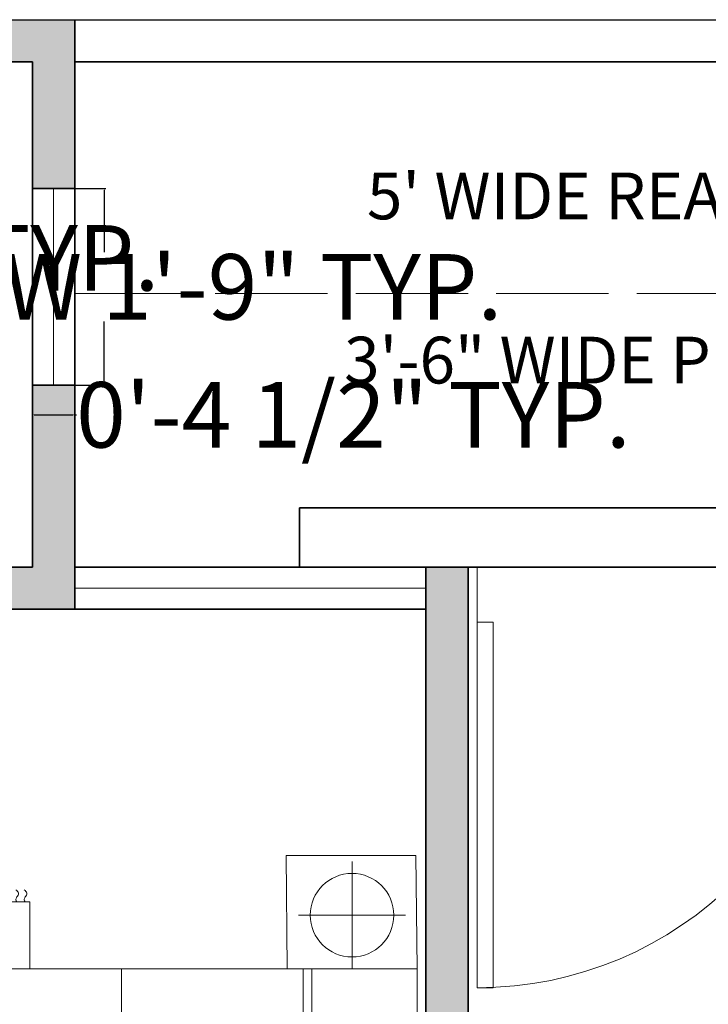
# Model space of a CAD drawing. Units: inches. Extents: x 0 to 4258, y 0 to 3769.
# Tile 23 of 30: x 3772 to 3845, y 3552 to 3657. Entities that reach past the tile are written whole.
import ezdxf

# ---------------------------------------------------------------- set-up
doc = ezdxf.new("R2010")
doc.units = ezdxf.units.IN
doc.header["$MEASUREMENT"] = 0
doc.linetypes.add('ACAD_ISO02W100', pattern=[15, 12, -3])
doc.layers.get('0').update_dxf_attribs({"color": 16})
for name, color, linetype, lineweight in [('A-ANNO-DIMS', 250, 'Continuous', 18), ('A-ANNO-TEXT', 250, 'Continuous', 18), ('A-FLOR-OVHD', 150, 'ACAD_ISO02W100', 13), ('A-WALL-PATT', 16, 'Continuous', 13), ('C-PROP', 150, 'Continuous', 25), ('doors', 250, 'Continuous', 18), ('furniture', 13, 'Continuous', 18), ('walls', 251, 'Continuous', 35), ('windows', 121, 'Continuous', 18)]:
    doc.layers.add(name, color=color, linetype=linetype, lineweight=lineweight)
doc.styles.get("Standard").update_dxf_attribs({"font": 'arial.ttf'})
doc.dimstyles.get("Standard").update_dxf_attribs({"dimtxt": 7, "dimasz": 0.18, "dimexe": 0.18, "dimexo": 0.0625, "dimgap": 0.09, "dimtad": 0, "dimtih": 1, "dimtoh": 1, "dimzin": 0, "dimdsep": 46, "dimlunit": 3, "dimtxsty": 'Standard', "dimcen": 0.09, "dimadec": 0, "dimazin": 0, "dimtfac": 1, "dimtofl": 0, "dimtmove": 0, "dimatfit": 3, "dimfxl": 1, "dimtolj": 1, "dimtzin": 0, "dimarcsym": 0})

# ---------------------------------------------------------------- blocks, each defined once
blk = doc.blocks.new('CARPET')
at = {"layer": 'furniture'}
for p, q in [((-51.53, -98.11), (-51.53, -55.12)), ((-51.53, -55.12), (-41.27, -55.12)), ((36, -55.12), (51.55, -55.12)), ((51.55, -55.12), (51.55, -98.11)), ((51.55, -98.11), (-51.53, -98.11))]:
    blk.add_line(p, q, dxfattribs=at)
for points, knots in [([(-53.37, -55.99), (-53.22, -55.8), (-52.9, -55.41), (-52.34, -55.8), (-51.89, -56.08), (-51.65, -55.91), (-51.53, -55.83)], [0, 0, 0, 0, 0.653278, 1.290138, 1.740457, 2.114451, 2.114451, 2.114451, 2.114451]), ([(53.37, -55.99), (53.22, -55.8), (52.9, -55.41), (52.34, -55.8), (51.89, -56.08), (51.65, -55.91), (51.53, -55.83)], [0, 0, 0, 0, 0.653278, 1.290138, 1.740457, 2.114451, 2.114451, 2.114451, 2.114451]), ([(-53.37, -57.26), (-53.22, -57.07), (-52.9, -56.67), (-52.34, -57.07), (-51.89, -57.35), (-51.65, -57.17), (-51.53, -57.1)], [0, 0, 0, 0, 0.653278, 1.290138, 1.740457, 2.114451, 2.114451, 2.114451, 2.114451]), ([(53.37, -57.26), (53.22, -57.07), (52.9, -56.67), (52.34, -57.07), (51.89, -57.35), (51.65, -57.17), (51.53, -57.1)], [0, 0, 0, 0, 0.653278, 1.290138, 1.740457, 2.114451, 2.114451, 2.114451, 2.114451]), ([(-53.37, -58.59), (-53.22, -58.4), (-52.9, -58.01), (-52.34, -58.4), (-51.89, -58.68), (-51.65, -58.5), (-51.53, -58.43)], [0, 0, 0, 0, 0.653278, 1.290138, 1.740457, 2.114451, 2.114451, 2.114451, 2.114451]), ([(53.37, -58.59), (53.22, -58.4), (52.9, -58.01), (52.34, -58.4), (51.89, -58.68), (51.65, -58.5), (51.53, -58.43)], [0, 0, 0, 0, 0.653278, 1.290138, 1.740457, 2.114451, 2.114451, 2.114451, 2.114451]), ([(-53.37, -59.78), (-53.22, -59.58), (-52.9, -59.19), (-52.34, -59.58), (-51.89, -59.86), (-51.65, -59.69), (-51.53, -59.61)], [0, 0, 0, 0, 0.653278, 1.290138, 1.740457, 2.114451, 2.114451, 2.114451, 2.114451]), ([(53.37, -59.78), (53.22, -59.58), (52.9, -59.19), (52.34, -59.58), (51.89, -59.86), (51.65, -59.69), (51.53, -59.61)], [0, 0, 0, 0, 0.653278, 1.290138, 1.740457, 2.114451, 2.114451, 2.114451, 2.114451]), ([(-53.37, -61.22), (-53.22, -61.02), (-52.9, -60.63), (-52.34, -61.02), (-51.89, -61.3), (-51.65, -61.13), (-51.53, -61.05)], [0, 0, 0, 0, 0.653278, 1.290138, 1.740457, 2.114451, 2.114451, 2.114451, 2.114451]), ([(53.37, -61.22), (53.22, -61.02), (52.9, -60.63), (52.34, -61.02), (51.89, -61.3), (51.65, -61.13), (51.53, -61.05)], [0, 0, 0, 0, 0.653278, 1.290138, 1.740457, 2.114451, 2.114451, 2.114451, 2.114451]), ([(-53.37, -62.44), (-53.22, -62.25), (-52.9, -61.86), (-52.34, -62.25), (-51.89, -62.53), (-51.65, -62.36), (-51.53, -62.28)], [0, 0, 0, 0, 0.653278, 1.290138, 1.740457, 2.114451, 2.114451, 2.114451, 2.114451]), ([(-53.37, -63.63), (-53.22, -63.43), (-52.9, -63.04), (-52.34, -63.43), (-51.89, -63.72), (-51.65, -63.54), (-51.53, -63.46)], [0, 0, 0, 0, 0.653278, 1.290138, 1.740457, 2.114451, 2.114451, 2.114451, 2.114451]), ([(53.37, -62.44), (53.22, -62.25), (52.9, -61.86), (52.34, -62.25), (51.89, -62.53), (51.65, -62.36), (51.53, -62.28)], [0, 0, 0, 0, 0.653278, 1.290138, 1.740457, 2.114451, 2.114451, 2.114451, 2.114451]), ([(53.37, -63.63), (53.22, -63.43), (52.9, -63.04), (52.34, -63.43), (51.89, -63.72), (51.65, -63.54), (51.53, -63.46)], [0, 0, 0, 0, 0.653278, 1.290138, 1.740457, 2.114451, 2.114451, 2.114451, 2.114451]), ([(-53.37, -65.07), (-53.22, -64.87), (-52.9, -64.48), (-52.34, -64.87), (-51.89, -65.15), (-51.65, -64.98), (-51.53, -64.9)], [0, 0, 0, 0, 0.653278, 1.290138, 1.740457, 2.114451, 2.114451, 2.114451, 2.114451]), ([(53.37, -65.07), (53.22, -64.87), (52.9, -64.48), (52.34, -64.87), (51.89, -65.15), (51.65, -64.98), (51.53, -64.9)], [0, 0, 0, 0, 0.653278, 1.290138, 1.740457, 2.114451, 2.114451, 2.114451, 2.114451]), ([(-53.37, -66.76), (-53.22, -66.56), (-52.9, -66.17), (-52.34, -66.56), (-51.89, -66.84), (-51.65, -66.67), (-51.53, -66.59)], [0, 0, 0, 0, 0.653278, 1.290138, 1.740457, 2.114451, 2.114451, 2.114451, 2.114451]), ([(-53.37, -68.2), (-53.22, -68), (-52.9, -67.61), (-52.34, -68), (-51.89, -68.28), (-51.65, -68.11), (-51.53, -68.03)], [0, 0, 0, 0, 0.653278, 1.290138, 1.740457, 2.114451, 2.114451, 2.114451, 2.114451]), ([(53.37, -66.76), (53.22, -66.56), (52.9, -66.17), (52.34, -66.56), (51.89, -66.84), (51.65, -66.67), (51.53, -66.59)], [0, 0, 0, 0, 0.653278, 1.290138, 1.740457, 2.114451, 2.114451, 2.114451, 2.114451]), ([(53.37, -68.2), (53.22, -68), (52.9, -67.61), (52.34, -68), (51.89, -68.28), (51.65, -68.11), (51.53, -68.03)], [0, 0, 0, 0, 0.653278, 1.290138, 1.740457, 2.114451, 2.114451, 2.114451, 2.114451]), ([(-53.37, -69.53), (-53.22, -69.33), (-52.9, -68.94), (-52.34, -69.33), (-51.89, -69.61), (-51.65, -69.44), (-51.53, -69.36)], [0, 0, 0, 0, 0.653278, 1.290138, 1.740457, 2.114451, 2.114451, 2.114451, 2.114451]), ([(53.37, -69.53), (53.22, -69.33), (52.9, -68.94), (52.34, -69.33), (51.89, -69.61), (51.65, -69.44), (51.53, -69.36)], [0, 0, 0, 0, 0.653278, 1.290138, 1.740457, 2.114451, 2.114451, 2.114451, 2.114451]), ([(-53.37, -70.79), (-53.22, -70.6), (-52.9, -70.21), (-52.34, -70.6), (-51.89, -70.88), (-51.65, -70.7), (-51.53, -70.63)], [0, 0, 0, 0, 0.653278, 1.290138, 1.740457, 2.114451, 2.114451, 2.114451, 2.114451]), ([(53.37, -70.79), (53.22, -70.6), (52.9, -70.21), (52.34, -70.6), (51.89, -70.88), (51.65, -70.7), (51.53, -70.63)], [0, 0, 0, 0, 0.653278, 1.290138, 1.740457, 2.114451, 2.114451, 2.114451, 2.114451]), ([(-53.37, -72.12), (-53.22, -71.93), (-52.9, -71.54), (-52.34, -71.93), (-51.89, -72.21), (-51.65, -72.04), (-51.53, -71.96)], [0, 0, 0, 0, 0.653278, 1.290138, 1.740457, 2.114451, 2.114451, 2.114451, 2.114451]), ([(53.37, -72.12), (53.22, -71.93), (52.9, -71.54), (52.34, -71.93), (51.89, -72.21), (51.65, -72.04), (51.53, -71.96)], [0, 0, 0, 0, 0.653278, 1.290138, 1.740457, 2.114451, 2.114451, 2.114451, 2.114451]), ([(-53.37, -73.31), (-53.22, -73.11), (-52.9, -72.72), (-52.34, -73.11), (-51.89, -73.4), (-51.65, -73.22), (-51.53, -73.14)], [0, 0, 0, 0, 0.653278, 1.290138, 1.740457, 2.114451, 2.114451, 2.114451, 2.114451]), ([(53.37, -73.31), (53.22, -73.11), (52.9, -72.72), (52.34, -73.11), (51.89, -73.4), (51.65, -73.22), (51.53, -73.14)], [0, 0, 0, 0, 0.653278, 1.290138, 1.740457, 2.114451, 2.114451, 2.114451, 2.114451]), ([(-53.37, -74.75), (-53.22, -74.55), (-52.9, -74.16), (-52.34, -74.55), (-51.89, -74.83), (-51.65, -74.66), (-51.53, -74.58)], [0, 0, 0, 0, 0.653278, 1.290138, 1.740457, 2.114451, 2.114451, 2.114451, 2.114451]), ([(53.37, -74.75), (53.22, -74.55), (52.9, -74.16), (52.34, -74.55), (51.89, -74.83), (51.65, -74.66), (51.53, -74.58)], [0, 0, 0, 0, 0.653278, 1.290138, 1.740457, 2.114451, 2.114451, 2.114451, 2.114451]), ([(-53.37, -75.98), (-53.22, -75.78), (-52.9, -75.39), (-52.34, -75.78), (-51.89, -76.06), (-51.65, -75.89), (-51.53, -75.81)], [0, 0, 0, 0, 0.653278, 1.290138, 1.740457, 2.114451, 2.114451, 2.114451, 2.114451]), ([(-53.37, -77.16), (-53.22, -76.96), (-52.9, -76.57), (-52.34, -76.96), (-51.89, -77.25), (-51.65, -77.07), (-51.53, -76.99)], [0, 0, 0, 0, 0.653278, 1.290138, 1.740457, 2.114451, 2.114451, 2.114451, 2.114451]), ([(53.37, -75.98), (53.22, -75.78), (52.9, -75.39), (52.34, -75.78), (51.89, -76.06), (51.65, -75.89), (51.53, -75.81)], [0, 0, 0, 0, 0.653278, 1.290138, 1.740457, 2.114451, 2.114451, 2.114451, 2.114451]), ([(53.37, -77.16), (53.22, -76.96), (52.9, -76.57), (52.34, -76.96), (51.89, -77.25), (51.65, -77.07), (51.53, -76.99)], [0, 0, 0, 0, 0.653278, 1.290138, 1.740457, 2.114451, 2.114451, 2.114451, 2.114451]), ([(-53.37, -78.6), (-53.22, -78.4), (-52.9, -78.01), (-52.34, -78.4), (-51.89, -78.68), (-51.65, -78.51), (-51.53, -78.43)], [0, 0, 0, 0, 0.653278, 1.290138, 1.740457, 2.114451, 2.114451, 2.114451, 2.114451]), ([(53.37, -78.6), (53.22, -78.4), (52.9, -78.01), (52.34, -78.4), (51.89, -78.68), (51.65, -78.51), (51.53, -78.43)], [0, 0, 0, 0, 0.653278, 1.290138, 1.740457, 2.114451, 2.114451, 2.114451, 2.114451]), ([(-53.37, -80.29), (-53.22, -80.09), (-52.9, -79.7), (-52.34, -80.09), (-51.89, -80.37), (-51.65, -80.2), (-51.53, -80.12)], [0, 0, 0, 0, 0.653278, 1.290138, 1.740457, 2.114451, 2.114451, 2.114451, 2.114451]), ([(-53.37, -81.73), (-53.22, -81.53), (-52.9, -81.14), (-52.34, -81.53), (-51.89, -81.81), (-51.65, -81.64), (-51.53, -81.56)], [0, 0, 0, 0, 0.653278, 1.290138, 1.740457, 2.114451, 2.114451, 2.114451, 2.114451]), ([(53.37, -80.29), (53.22, -80.09), (52.9, -79.7), (52.34, -80.09), (51.89, -80.37), (51.65, -80.2), (51.53, -80.12)], [0, 0, 0, 0, 0.653278, 1.290138, 1.740457, 2.114451, 2.114451, 2.114451, 2.114451]), ([(53.37, -81.73), (53.22, -81.53), (52.9, -81.14), (52.34, -81.53), (51.89, -81.81), (51.65, -81.64), (51.53, -81.56)], [0, 0, 0, 0, 0.653278, 1.290138, 1.740457, 2.114451, 2.114451, 2.114451, 2.114451]), ([(-53.37, -83.06), (-53.22, -82.86), (-52.9, -82.47), (-52.34, -82.86), (-51.89, -83.14), (-51.65, -82.97), (-51.53, -82.89)], [0, 0, 0, 0, 0.653278, 1.290138, 1.740457, 2.114451, 2.114451, 2.114451, 2.114451]), ([(53.37, -83.06), (53.22, -82.86), (52.9, -82.47), (52.34, -82.86), (51.89, -83.14), (51.65, -82.97), (51.53, -82.89)], [0, 0, 0, 0, 0.653278, 1.290138, 1.740457, 2.114451, 2.114451, 2.114451, 2.114451]), ([(-53.37, -84.18), (-53.22, -83.99), (-52.9, -83.6), (-52.34, -83.99), (-51.89, -84.27), (-51.65, -84.09), (-51.53, -84.02)], [0, 0, 0, 0, 0.653278, 1.290138, 1.740457, 2.114451, 2.114451, 2.114451, 2.114451]), ([(53.37, -84.18), (53.22, -83.99), (52.9, -83.6), (52.34, -83.99), (51.89, -84.27), (51.65, -84.09), (51.53, -84.02)], [0, 0, 0, 0, 0.653278, 1.290138, 1.740457, 2.114451, 2.114451, 2.114451, 2.114451]), ([(-53.37, -85.51), (-53.22, -85.32), (-52.9, -84.93), (-52.34, -85.32), (-51.89, -85.6), (-51.65, -85.42), (-51.53, -85.35)], [0, 0, 0, 0, 0.653278, 1.290138, 1.740457, 2.114451, 2.114451, 2.114451, 2.114451]), ([(53.37, -85.51), (53.22, -85.32), (52.9, -84.93), (52.34, -85.32), (51.89, -85.6), (51.65, -85.42), (51.53, -85.35)], [0, 0, 0, 0, 0.653278, 1.290138, 1.740457, 2.114451, 2.114451, 2.114451, 2.114451]), ([(-53.37, -86.7), (-53.22, -86.5), (-52.9, -86.11), (-52.34, -86.5), (-51.89, -86.78), (-51.65, -86.61), (-51.53, -86.53)], [0, 0, 0, 0, 0.653278, 1.290138, 1.740457, 2.114451, 2.114451, 2.114451, 2.114451]), ([(53.37, -86.7), (53.22, -86.5), (52.9, -86.11), (52.34, -86.5), (51.89, -86.78), (51.65, -86.61), (51.53, -86.53)], [0, 0, 0, 0, 0.653278, 1.290138, 1.740457, 2.114451, 2.114451, 2.114451, 2.114451]), ([(-53.37, -88.14), (-53.22, -87.94), (-52.9, -87.55), (-52.34, -87.94), (-51.89, -88.22), (-51.65, -88.05), (-51.53, -87.97)], [0, 0, 0, 0, 0.653278, 1.290138, 1.740457, 2.114451, 2.114451, 2.114451, 2.114451]), ([(53.37, -88.14), (53.22, -87.94), (52.9, -87.55), (52.34, -87.94), (51.89, -88.22), (51.65, -88.05), (51.53, -87.97)], [0, 0, 0, 0, 0.653278, 1.290138, 1.740457, 2.114451, 2.114451, 2.114451, 2.114451]), ([(-53.37, -89.36), (-53.22, -89.17), (-52.9, -88.78), (-52.34, -89.17), (-51.89, -89.45), (-51.65, -89.28), (-51.53, -89.2)], [0, 0, 0, 0, 0.653278, 1.290138, 1.740457, 2.114451, 2.114451, 2.114451, 2.114451]), ([(-53.37, -90.55), (-53.22, -90.35), (-52.9, -89.96), (-52.34, -90.35), (-51.89, -90.64), (-51.65, -90.46), (-51.53, -90.38)], [0, 0, 0, 0, 0.653278, 1.290138, 1.740457, 2.114451, 2.114451, 2.114451, 2.114451]), ([(53.37, -89.36), (53.22, -89.17), (52.9, -88.78), (52.34, -89.17), (51.89, -89.45), (51.65, -89.28), (51.53, -89.2)], [0, 0, 0, 0, 0.653278, 1.290138, 1.740457, 2.114451, 2.114451, 2.114451, 2.114451]), ([(53.37, -90.55), (53.22, -90.35), (52.9, -89.96), (52.34, -90.35), (51.9, -90.63), (51.66, -90.47), (51.55, -90.4)], [0, 0, 0, 0, 0.653278, 1.290138, 1.740457, 2.0926, 2.0926, 2.0926, 2.0926]), ([(-53.37, -91.99), (-53.22, -91.79), (-52.9, -91.4), (-52.34, -91.79), (-51.89, -92.07), (-51.65, -91.9), (-51.53, -91.82)], [0, 0, 0, 0, 0.653278, 1.290138, 1.740457, 2.114451, 2.114451, 2.114451, 2.114451]), ([(53.37, -91.99), (53.22, -91.79), (52.9, -91.4), (52.34, -91.79), (51.9, -92.07), (51.66, -91.91), (51.55, -91.83)], [0, 0, 0, 0, 0.653278, 1.290138, 1.740457, 2.0926, 2.0926, 2.0926, 2.0926]), ([(-53.37, -92.69), (-53.22, -92.48), (-52.9, -92.08), (-52.35, -92.49), (-51.89, -92.77), (-51.65, -92.6), (-51.53, -92.52)], [0, 0, 0, 0, 0.663904, 1.307406, 1.757725, 2.131719, 2.131719, 2.131719, 2.131719]), ([(-53.37, -93.61), (-53.22, -93.42), (-52.9, -93.03), (-52.34, -93.42), (-51.89, -93.7), (-51.65, -93.52), (-51.53, -93.45)], [0, 0, 0, 0, 0.653278, 1.290138, 1.740457, 2.114451, 2.114451, 2.114451, 2.114451]), ([(53.37, -92.69), (53.22, -92.49), (52.9, -92.09), (52.34, -92.49), (51.9, -92.77), (51.66, -92.61), (51.55, -92.53)], [0, 0, 0, 0, 0.656792, 1.295826, 1.746145, 2.098292, 2.098292, 2.098292, 2.098292]), ([(53.37, -93.66), (53.22, -93.46), (52.9, -93.07), (52.34, -93.46), (51.9, -93.74), (51.66, -93.58), (51.55, -93.5)], [0, 0, 0, 0, 0.653278, 1.290138, 1.740457, 2.0926, 2.0926, 2.0926, 2.0926]), ([(-53.37, -94.55), (-53.22, -94.35), (-52.9, -93.96), (-52.34, -94.35), (-51.89, -94.63), (-51.65, -94.46), (-51.53, -94.38)], [0, 0, 0, 0, 0.653278, 1.290138, 1.740457, 2.114451, 2.114451, 2.114451, 2.114451]), ([(-53.37, -95.05), (-53.22, -94.85), (-52.9, -94.46), (-52.34, -94.85), (-51.89, -95.14), (-51.65, -94.96), (-51.53, -94.88)], [0, 0, 0, 0, 0.653278, 1.290138, 1.740457, 2.114451, 2.114451, 2.114451, 2.114451]), ([(53.37, -94.59), (53.22, -94.4), (52.9, -94.01), (52.34, -94.4), (51.9, -94.68), (51.66, -94.51), (51.55, -94.44)], [0, 0, 0, 0, 0.653278, 1.290138, 1.740457, 2.0926, 2.0926, 2.0926, 2.0926]), ([(53.37, -95.1), (53.22, -94.9), (52.9, -94.51), (52.34, -94.9), (51.9, -95.18), (51.66, -95.02), (51.55, -94.94)], [0, 0, 0, 0, 0.653278, 1.290138, 1.740457, 2.0926, 2.0926, 2.0926, 2.0926]), ([(-53.37, -95.73), (-53.22, -95.54), (-52.9, -95.15), (-52.34, -95.54), (-51.89, -95.82), (-51.65, -95.65), (-51.53, -95.57)], [0, 0, 0, 0, 0.653278, 1.290138, 1.740457, 2.114451, 2.114451, 2.114451, 2.114451]), ([(-53.37, -96.38), (-53.22, -96.18), (-52.9, -95.79), (-52.34, -96.18), (-51.89, -96.47), (-51.65, -96.29), (-51.53, -96.21)], [0, 0, 0, 0, 0.653278, 1.290138, 1.740457, 2.114451, 2.114451, 2.114451, 2.114451]), ([(53.37, -95.78), (53.22, -95.58), (52.9, -95.19), (52.34, -95.58), (51.89, -95.86), (51.65, -95.69), (51.53, -95.61)], [0, 0, 0, 0, 0.653278, 1.290138, 1.740457, 2.114451, 2.114451, 2.114451, 2.114451]), ([(53.37, -96.43), (53.22, -96.23), (52.9, -95.84), (52.34, -96.23), (51.89, -96.51), (51.65, -96.34), (51.53, -96.26)], [0, 0, 0, 0, 0.653278, 1.290138, 1.740457, 2.114451, 2.114451, 2.114451, 2.114451]), ([(-53.37, -97.17), (-53.22, -96.98), (-52.9, -96.59), (-52.34, -96.98), (-51.89, -97.26), (-51.65, -97.08), (-51.53, -97.01)], [0, 0, 0, 0, 0.653278, 1.290138, 1.740457, 2.114451, 2.114451, 2.114451, 2.114451]), ([(-53.37, -97.99), (-53.22, -97.79), (-52.9, -97.4), (-52.34, -97.79), (-51.89, -98.08), (-51.65, -97.9), (-51.53, -97.82)], [0, 0, 0, 0, 0.653278, 1.290138, 1.740457, 2.114451, 2.114451, 2.114451, 2.114451]), ([(53.37, -97.22), (53.22, -97.02), (52.9, -96.63), (52.34, -97.02), (51.89, -97.3), (51.65, -97.13), (51.53, -97.05)], [0, 0, 0, 0, 0.653278, 1.290138, 1.740457, 2.114451, 2.114451, 2.114451, 2.114451]), ([(53.37, -97.99), (53.22, -97.79), (52.9, -97.4), (52.34, -97.79), (51.89, -98.08), (51.65, -97.9), (51.53, -97.82)], [0, 0, 0, 0, 0.653278, 1.290138, 1.740457, 2.114451, 2.114451, 2.114451, 2.114451])]:
    blk.add_open_spline(points, degree=3, knots=knots, dxfattribs=at)
blk = doc.blocks.new('A$C58D270C6')
at = {"layer": 'furniture'}
for p, q in [((9.09, 124.13), (9.09, 108.87)), ((1.46, 116.5), (16.73, 116.5)), ((14.97, 94.84), (24.62, 107.92)), ((24.62, 94.93), (24.62, 107.92)), ((42.08, 108), (42.08, 36)), ((14.97, 94.93), (24.62, 94.93)), ((14.97, 94.84), (14.97, 36)), ((16.22, 94.93), (16.22, 36)), ((9.25, 36), (9.25, 20.74)), ((1.62, 28.37), (16.88, 28.37))]:
    blk.add_line(p, q, dxfattribs=at)
for points in [[(18.5, 108), (18.34, 124.13), (-0.16, 124.13), (0, 108)], [(0, 108), (77.91, 108), (77.91, 36), (0, 36)], [(4.09, 94.93), (14.97, 94.93), (14.97, 73.83), (4.09, 73.83)], [(4.09, 65.23), (14.97, 65.23), (14.97, 44.13), (4.09, 44.13)], [(18.65, 19.87), (18.5, 36), (0, 36), (0.16, 19.87)]]:
    blk.add_lwpolyline(points, close=True, dxfattribs=at)
for centre in [(9.09, 116.5), (9.25, 28.37)]:
    blk.add_circle(centre, 5.95, dxfattribs=at)
at = {"layer": 'furniture', "xscale": 0.9312884925094044, "yscale": 0.9312884925094044, "zscale": 0.9312884925094044, "rotation": 90}
blk.add_blockref('CARPET', (3.79, 74.47), dxfattribs=at)
blk = doc.blocks.new('*U23')
for p, q in [((0, 0), (0, -6)), ((40, 0), (40, -6))]:
    blk.add_line(p, q)
blk.add_lwpolyline([(0, 0), (0, 40), (1.75, 40), (1.75, 0)], close=True)
blk.add_arc((0, 0), 40, 0, 90)
blk = doc.blocks.new('WINDOW-21IN')
for p, q in [((0, 21.04), (0, 0)), ((2.25, 21.04), (2.25, 0)), ((4.5, 21.04), (4.5, 0))]:
    blk.add_line(p, q)
blk = doc.blocks.new('*D54')
at = {"layer": 'A-ANNO-DIMS', "color": 0, "lineweight": -2, "transparency": 16777216}
for p, q in [((3684.72, 3634.74), (3684.72, 3631.16)), ((3707.82, 3634.74), (3707.82, 3631.16)), ((3684.9, 3631.34), (3707.64, 3631.34)), ((3707.82, 3631.34), (3708, 3631.34))]:
    blk.add_line(p, q, dxfattribs=at)
at = {"layer": 'A-ANNO-DIMS', "color": 0, "transparency": 16777216}
for points in [[(3684.9, 3631.37), (3684.9, 3631.31), (3684.72, 3631.34)], [(3707.64, 3631.37), (3707.64, 3631.31), (3707.82, 3631.34)]]:
    blk.add_solid(points, dxfattribs=at)
at = {"layer": 'Defpoints', "color": 0, "transparency": 16777216}
for p in [(3684.72, 3634.8), (3707.82, 3634.8), (3707.82, 3631.34)]:
    blk.add_point(p, dxfattribs=at)
at = {"layer": 'A-ANNO-DIMS', "color": 0, "transparency": 16777216, "insert": (3748.02, 3631.34), "char_height": 7, "attachment_point": 5}
blk.add_mtext('\\A1;BASIN 1\'-11" TYP.', dxfattribs=at)
blk = doc.blocks.new('*D62')
at = {"layer": 'A-ANNO-DIMS', "color": 0, "lineweight": -2, "transparency": 16777216}
for p, q in [((3777.87, 3638.77), (3781.14, 3638.77)), ((3780.96, 3638.59), (3780.96, 3631.96)), ((3780.96, 3617.91), (3780.96, 3624.54)), ((3777.87, 3617.73), (3781.14, 3617.73))]:
    blk.add_line(p, q, dxfattribs=at)
at = {"layer": 'A-ANNO-DIMS', "color": 0, "transparency": 16777216}
for points in [[(3780.93, 3638.59), (3780.99, 3638.59), (3780.96, 3638.77)], [(3780.93, 3617.91), (3780.99, 3617.91), (3780.96, 3617.73)]]:
    blk.add_solid(points, dxfattribs=at)
at = {"layer": 'Defpoints', "color": 0, "transparency": 16777216}
for p in [(3777.8, 3638.77), (3780.96, 3638.77), (3777.8, 3617.73)]:
    blk.add_point(p, dxfattribs=at)
at = {"layer": 'A-ANNO-DIMS', "color": 0, "transparency": 16777216, "insert": (3780.96, 3628.25), "char_height": 7, "attachment_point": 5}
blk.add_mtext('\\A1;WINDOW 1\'-9" TYP.', dxfattribs=at)
blk = doc.blocks.new('*D63')
at = {"layer": 'A-ANNO-DIMS', "color": 0, "lineweight": -2, "transparency": 16777216}
for p, q in [((3773.3, 3617.67), (3773.3, 3614.39)), ((3777.8, 3617.67), (3777.8, 3614.39)), ((3773.48, 3614.57), (3777.62, 3614.57)), ((3777.8, 3614.57), (3777.98, 3614.57))]:
    blk.add_line(p, q, dxfattribs=at)
at = {"layer": 'A-ANNO-DIMS', "color": 0, "transparency": 16777216}
for points in [[(3773.48, 3614.6), (3773.48, 3614.54), (3773.3, 3614.57)], [(3777.62, 3614.6), (3777.62, 3614.54), (3777.8, 3614.57)]]:
    blk.add_solid(points, dxfattribs=at)
at = {"layer": 'Defpoints', "color": 0, "transparency": 16777216}
for p in [(3773.3, 3617.73), (3777.8, 3617.73), (3777.8, 3614.57)]:
    blk.add_point(p, dxfattribs=at)
at = {"layer": 'A-ANNO-DIMS', "color": 0, "transparency": 16777216, "insert": (3807.56, 3614.57), "char_height": 7, "attachment_point": 5}
blk.add_mtext('\\A1;0\'-4 1/2" TYP.', dxfattribs=at)

msp = doc.modelspace()

# ---------------------------------------------------------------- hatches: boundary and pattern name
at = {"layer": 'A-WALL-PATT'}
h = msp.add_hatch(color=256, dxfattribs=at)
h.dxf.hatch_style = 1
h.paths.add_polyline_path([(3753.804, 3425.793), (3753.804, 3437.642), (3815.304, 3437.642), (3815.304, 3421.293), (3819.804, 3421.293), (3819.804, 3442.142), (3749.304, 3442.142), (3749.304, 3425.793), (3683.304, 3425.793), (3683.304, 3652.293), (3773.304, 3652.293), (3773.304, 3638.769), (3777.804, 3638.769), (3777.804, 3656.793), (3678.804, 3656.793), (3678.804, 3163.293), (3711.393, 3163.293), (3711.393, 3167.793), (3683.304, 3167.793), (3683.304, 3374.793), (3693.303, 3374.793), (3693.303, 3379.293), (3683.304, 3379.293), (3683.304, 3421.293), (3749.304, 3421.293), (3749.304, 3379.293), (3741.449, 3379.293), (3741.449, 3374.793), (3753.804, 3374.793)])
h = msp.add_hatch(color=256, dxfattribs=at)
h.dxf.hatch_style = 1
h.paths.add_polyline_path([(3777.804, 3598.293), (3777.804, 3617.728), (3773.304, 3617.728), (3773.304, 3598.293), (3708.48, 3598.293), (3708.48, 3593.793), (3777.804, 3593.793)])
h = msp.add_hatch(color=256, dxfattribs=at)
h.dxf.hatch_style = 1
h.paths.add_polyline_path([(3777.804, 3598.293), (3777.804, 3617.728), (3773.304, 3617.728), (3773.304, 3598.293), (3708.48, 3598.293), (3708.48, 3593.793), (3777.804, 3593.793)])
h = msp.add_hatch(color=256, dxfattribs=at)
h.dxf.hatch_style = 1
h.paths.add_polyline_path([(3819.804, 3598.293), (3815.304, 3598.293), (3815.304, 3487.182), (3819.804, 3487.182)])

# ---------------------------------------------------------------- linework, layer by layer
at = {"layer": 'A-FLOR-OVHD'}
msp.add_line((3777.804, 3627.543), (3933.804, 3627.543), dxfattribs=at)
at = {"layer": 'C-PROP'}
for p, q in [((3678.804, 3656.793), (4038.804, 3656.793)), ((3777.804, 3656.793), (3933.804, 3656.793)), ((3777.804, 3652.293), (3933.804, 3652.293))]:
    msp.add_line(p, q, dxfattribs=at)
at = {"layer": 'walls'}
for p, q in [((3777.804, 3598.293), (3777.804, 3656.793)), ((3683.304, 3652.293), (3773.304, 3652.293)), ((3773.304, 3598.293), (3773.304, 3652.293)), ((3777.804, 3652.293), (3933.804, 3652.293)), ((3777.804, 3638.769), (3773.304, 3638.769)), ((3777.804, 3617.728), (3773.304, 3617.728)), ((3801.818, 3598.293), (3801.818, 3604.636)), ((3801.818, 3604.636), (3874.654, 3604.636)), ((3708.47, 3598.293), (3773.304, 3598.293)), ((3777.804, 3598.293), (3819.804, 3598.293)), ((3777.804, 3598.293), (3777.804, 3593.793)), ((3815.304, 3487.182), (3815.304, 3598.293)), ((3819.804, 3421.293), (3819.804, 3598.293)), ((3819.804, 3598.293), (3861.804, 3598.293)), ((3683.304, 3593.793), (3815.304, 3593.793))]:
    msp.add_line(p, q, dxfattribs=at)
at = {"layer": 'windows'}
for p, q in [((3815.304, 3598.293), (3777.804, 3598.293)), ((3815.304, 3596.043), (3777.804, 3596.043)), ((3815.304, 3593.793), (3777.804, 3593.793))]:
    msp.add_line(p, q, dxfattribs=at)

# ---------------------------------------------------------------- block references
at = {"layer": 'doors', "xscale": -0.9769813032789267, "yscale": 0.9769813032789267, "zscale": 0.9769813032789267, "rotation": 180}
msp.add_blockref('*U23', (3820.752, 3592.431), dxfattribs=at)
at = {"layer": 'furniture', "xscale": 0.7500000390647866, "yscale": 0.7500000390647866, "zscale": 0.7500000390647866, "rotation": 180}
msp.add_blockref('A$C58D270C6', (3814.348, 3582.385), dxfattribs=at)
at = {"layer": 'windows'}
msp.add_blockref('WINDOW-21IN', (3773.304, 3617.728), dxfattribs=at)

# ---------------------------------------------------------------- texts
at = {"layer": 'A-ANNO-TEXT'}
for s, p in [("5' WIDE REAR SET BACK", (3808.998, 3635.463)), ('3\'-6" WIDE PROJECTION', (3806.567, 3617.92))]:
    msp.add_text(s, height=5, dxfattribs=at).set_placement(p)

# ---------------------------------------------------------------- dimensions: what is measured, and where the dimension line sits
at = {"layer": 'A-ANNO-DIMS'}
for base, p1, p2, text, picture, middle in [((3707.824, 3631.338), (3684.717, 3634.804), (3707.824, 3634.804), 'BASIN <> TYP.', '*D54', (3748.024, 3631.338)), ((3777.804, 3614.572), (3773.304, 3617.728), (3777.804, 3617.728), '<> TYP.', '*D63', (3807.563, 3614.572))]:
    dim = msp.add_linear_dim(base=base, p1=p1, p2=p2, text=text, dimstyle='Standard', override={"dimdec": 1, "dimlfac": 1, "dimrnd": 0, "dimzin": 1, "dimdsep": 46, "dimlunit": 4, "dimfrac": 2}, dxfattribs=at)
    dim.commit()
    dim.dimension.update_dxf_attribs({"geometry": picture, "text_midpoint": middle})
dim = msp.add_linear_dim(base=(3780.96, 3638.769), p1=(3777.804, 3617.728), p2=(3777.804, 3638.769), angle=90, text='WINDOW <> TYP.', dimstyle='Standard', override={"dimdec": 1, "dimlfac": 1, "dimrnd": 0, "dimzin": 1, "dimdsep": 46, "dimlunit": 4, "dimfrac": 2}, dxfattribs=at)
dim.commit()
dim.dimension.update_dxf_attribs({"geometry": '*D62', "text_midpoint": (3780.96, 3628.249)})

doc.saveas('drawing.dxf')
